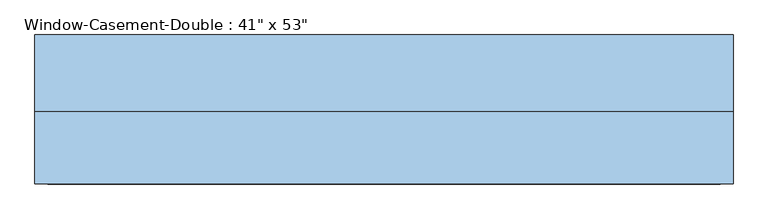
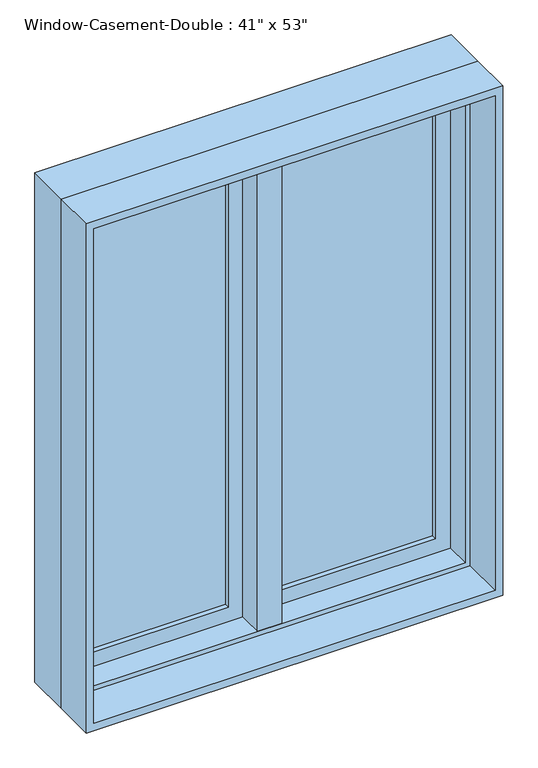
"""IFC4 building model written with IfcOpenShell, lengths in millimetres: window geometry."""

from ifc_helpers import new_model, si_unit, frame, origin, place, context, project, spatial, polyline, outline, extrude, faceted_brep, source, transform, mapped, element, save


def window_0de3df1e(model_context):
    return source(origin(), model_context, "Body", "SolidModel", [
        faceted_brep([(9.525, 120.65, 2247.9), (-9.525, 120.65, 2247.9), (-9.525, 69.85, 2247.9), (9.525, 69.85, 2247.9), (9.525, 120.65, 927.1), (9.525, 69.85, 927.1), (-9.525, 69.85, 927.1), (-9.525, 120.65, 927.1), (-9.525, 69.85, 946.15), (-9.525, 69.85, 2228.85), (-30.1625, 69.85, 946.15), (-30.1625, 69.85, 2228.85), (-30.1625, 6.35, 946.15), (-30.1625, 6.35, 2228.85), (30.1625, 6.35, 946.15), (30.1625, 6.35, 2228.85), (30.1625, 69.85, 946.15), (30.1625, 69.85, 2228.85), (9.525, 69.85, 946.15), (9.525, 69.85, 2228.85)], [[[0, 1, 2, 3]], [[4, 5, 6, 7]], [[1, 0, 4, 7]], [[2, 1, 7, 6, 8, 9]], [[9, 8, 10, 11]], [[11, 10, 12, 13]], [[13, 12, 14, 15]], [[15, 14, 16, 17]], [[17, 16, 18, 19]], [[0, 3, 19, 18, 5, 4]], [[18, 8, 6, 5]], [[9, 19, 3, 2]], [[8, 18, 16, 14, 12, 10]], [[19, 9, 11, 13, 15, 17]]]),
        extrude(outline(polyline([(-66.675, 101.6), (-66.675, 95.25), (-450.85, 95.25), (-450.85, 101.6), (-66.675, 101.6)])), frame((0.0, 0.0, 984.25), z_axis=(0.0, 0.0, 1.0), x_axis=(1.0, 0.0, 0.0)), (0.0, 0.0, 1.0), 1206.5),
        extrude(outline(polyline([(-450.85, 82.55), (-450.85, 88.9), (-66.675, 88.9), (-66.675, 82.55), (-450.85, 82.55)])), frame((0.0, 0.0, 984.25), z_axis=(0.0, 0.0, 1.0), x_axis=(1.0, 0.0, 0.0)), (0.0, 0.0, 1.0), 1206.5),
        extrude(outline(polyline([(450.85, 101.6), (450.85, 95.25), (66.675, 95.25), (66.675, 101.6), (450.85, 101.6)])), frame((0.0, 0.0, 984.25), z_axis=(0.0, 0.0, 1.0), x_axis=(1.0, 0.0, 0.0)), (0.0, 0.0, 1.0), 1206.5),
        extrude(outline(polyline([(66.675, 82.55), (66.675, 88.9), (450.85, 88.9), (450.85, 82.55), (66.675, 82.55)])), frame((0.0, 0.0, 984.25), z_axis=(0.0, 0.0, 1.0), x_axis=(1.0, 0.0, 0.0)), (0.0, 0.0, 1.0), 1206.5),
        extrude(outline(polyline([(2247.9, -508.0), (927.1, -508.0), (927.1, -9.525), (2247.9, -9.525), (2247.9, -508.0)]), holes=[polyline([(2190.75, -66.675), (984.25, -66.675), (984.25, -450.85), (2190.75, -450.85), (2190.75, -66.675)])]), frame((0.0, 69.85, 0.0), z_axis=(0.0, 1.0, 0.0), x_axis=(0.0, 0.0, 1.0)), (0.0, 0.0, 1.0), 44.45),
        extrude(outline(polyline([(927.1, 508.0), (2247.9, 508.0), (2247.9, 9.525), (927.1, 9.525), (927.1, 508.0)]), holes=[polyline([(984.25, 66.675), (2190.75, 66.675), (2190.75, 450.85), (984.25, 450.85), (984.25, 66.675)])]), frame((0.0, 69.85, 0.0), z_axis=(0.0, 1.0, 0.0), x_axis=(0.0, 0.0, 1.0)), (0.0, 0.0, 1.0), 44.45),
        extrude(outline(polyline([(2260.6, -520.7), (914.4, -520.7), (914.4, 520.7), (2260.6, 520.7), (2260.6, -520.7)]), holes=[polyline([(2241.55, 501.65), (933.45, 501.65), (933.45, -501.65), (2241.55, -501.65), (2241.55, 501.65)])]), frame((0.0, -101.6, 0.0), z_axis=(0.0, 1.0, 0.0), x_axis=(0.0, 0.0, 1.0)), (0.0, 0.0, 1.0), 107.95),
        faceted_brep([(488.95, 69.85, 2228.85), (488.95, 6.35, 2228.85), (-488.95, 6.35, 2228.85), (-488.95, 69.85, 2228.85), (508.0, 120.65, 2247.9), (508.0, 69.85, 2247.9), (-508.0, 69.85, 2247.9), (-508.0, 120.65, 2247.9), (520.7, 6.35, 2260.6), (520.7, 120.65, 2260.6), (-520.7, 120.65, 2260.6), (-520.7, 6.35, 2260.6), (-488.95, 6.35, 946.15), (-488.95, 69.85, 946.15), (-508.0, 69.85, 927.1), (-508.0, 120.65, 927.1), (-520.7, 120.65, 914.4), (-520.7, 6.35, 914.4), (488.95, 6.35, 946.15), (488.95, 69.85, 946.15), (508.0, 69.85, 927.1), (508.0, 120.65, 927.1), (520.7, 120.65, 914.4), (520.7, 6.35, 914.4)], [[[0, 1, 2, 3]], [[4, 5, 6, 7]], [[8, 9, 10, 11]], [[3, 2, 12, 13]], [[7, 6, 14, 15]], [[11, 10, 16, 17]], [[13, 12, 18, 19]], [[15, 14, 20, 21]], [[17, 16, 22, 23]], [[11, 17, 23, 8], [1, 18, 12, 2]], [[19, 18, 1, 0]], [[5, 20, 14, 6], [3, 13, 19, 0]], [[21, 20, 5, 4]], [[23, 22, 9, 8]], [[9, 22, 16, 10], [7, 15, 21, 4]]]),
    ])


if __name__ == "__main__":
    model = new_model("IFC4")
    model_context = context("Model", 3, world=origin())
    ifc_project = project(units=[si_unit("LENGTHUNIT", "METRE", prefix="MILLI")], contexts=[model_context])
    site = spatial("IfcSite", under=ifc_project)
    building = spatial("IfcBuilding", under=site)
    placement = place(None, origin())
    window_shape = window_0de3df1e(model_context)
    element("IfcWindow", 1, ObjectType="Window-Casement-Double : 41\" x 53\"", at=placement, inside=building, context=model_context, shape_type="MappedRepresentation", body=[
        mapped(window_shape, transform((0.0, 0.0, 0.0), x_axis=(1.0, 0.0, 0.0), y_axis=(0.0, 1.0, 0.0), z_axis=(0.0, 0.0, 1.0))),
    ])
    save(model, "model.ifc")

# Revit data of these elements
# Type "Window-Casement-Double : 41\" x 53\""
#   Type Mark = "15"
#   Fire Rating = "0.5h"
#   Assembly Code = "B2020100"
#   Analytic Construction = "Double glazing - domestic"
#   Frame Extension [instance default] = 0' - 0 1/4"
#   Window Inset [instance default] = 0' - 0"
#   Wall Thickness [instance default] = 0' - 6"
#   Interior Wall Closure [instance default] = 0' - 2 1/4"
#   Half Width = 1' - 8 1/2"
#   Visual Light Transmittance = 0.81
#   Thermal Resistance (R) = 1.8146 (h·ft²·°F)/BTU
#   Solar Heat Gain Coefficient = 0.76
#   Rough Width = 3' - 5 1/2"
#   Rough Height = 4' - 5 1/2"
#   Height = 4' - 5"
#   Heat Transfer Coefficient (U) = 0.5511 BTU/(h·ft²·°F)
#   Exterior Wall Closure [instance default] = 0' - 1 1/4"
#   Extension Jamb [instance default] = 0' - 2 1/4"
#   Default Sill Height = 3' - 0"
#   Width = 3' - 5"
#   Define Thermal Properties by = 0
#   Muntin Visibility = yes
#   Interior Trim Visibility [instance default] = yes
#   Exterior Trim Visibility [instance default] = yes
#   Extension Jamb Visibility [instance default] = yes
#   Interior Trim Material = Wood - Stained
#   Muntin Pattern = Muntin Pattern_2x2 : Muntin Pattern_2x2
#   Interior Trim = Trim-Window-Interior-Flat : Picture Frame
#   Interior Frame Material = Wood - Stained
#   Glass Panel Material = Glass
#   Exterior Trim Material = Clad - White
#   Exterior Trim = Trim-Window-Exterior-Flat : with Sill
#   Exterior Frame Material = Clad - White
#   Wall Closure = (empty or 0)
# Element 1 (IfcWindow, "Window-Casement-Double : 41\" x 53\"")
#   Wall Thickness = 0' - 8"
#   Extension Jamb = 0' - 4 1/4"
#   Materials on its faces: "Wood - Stained", "Glass", "Clad - White"
# Materials
#   "Wood - Stained": class "Wood", colour RGB 224 178 126, transparency 0, Cost = 0
#   "Glass": class "Glass", colour RGB 0 128 192, transparency 0.75, Description = "Soda Lime Glass", Cost = 0
#   "Clad - White": class "Wood", colour RGB 242 242 238, transparency 0, Cost = 0
